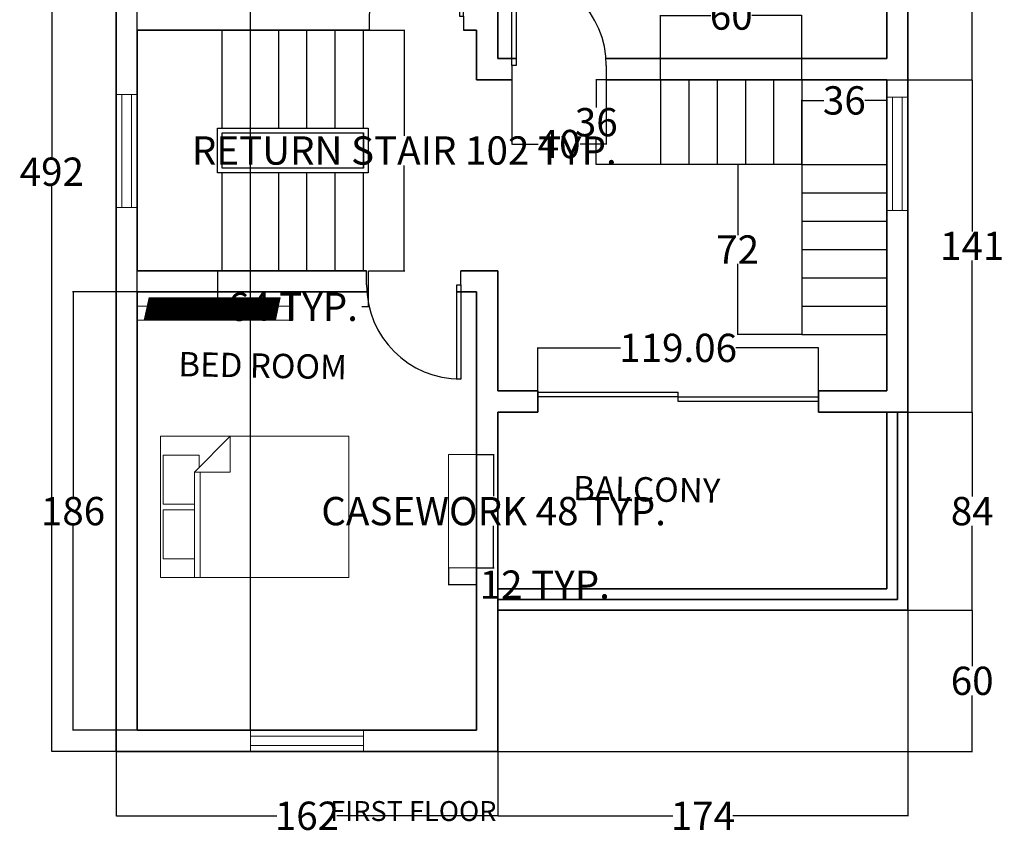
# Model space of a CAD drawing. Units: inches. Extents: x 424 to 1593, y 6 to 578.
# Tile 3 of 4: x 1175 to 1593, y 15 to 361. Entities that reach past the tile are written whole.
import ezdxf

# ---------------------------------------------------------------- set-up
doc = ezdxf.new("R2010")
doc.units = ezdxf.units.IN
doc.header["$MEASUREMENT"] = 0
for name, color, linetype, lineweight in [('A-ANNO-DIMS', 2, 'Continuous', 18), ('A-ANNO-TEXT', 7, 'Continuous', 25), ('A-AREA-IDEN', 7, 'Continuous', 18), ('A-DOOR', 3, 'Continuous', 25), ('A-FLOR-CASE', 9, 'Continuous', 18), ('A-FLOR-CASE-PATT', 252, 'Continuous', 13), ('A-FLOR-STRS', 7, 'Continuous', 25), ('A-FURN', 8, 'Continuous', 18), ('A-GLAZ', 4, 'Continuous', 18), ('A-WALL', 7, 'Continuous', 35)]:
    doc.layers.add(name, color=color, linetype=linetype, lineweight=lineweight)
doc.styles.get("Standard").update_dxf_attribs({"font": 'arial.ttf'})
doc.dimstyles.get("Standard").update_dxf_attribs({"dimtxt": 12, "dimasz": 0.18, "dimexe": 0.18, "dimexo": 0.0625, "dimgap": 0.09, "dimtad": 0, "dimtih": 1, "dimtoh": 1, "dimdec": 0, "dimzin": 0, "dimdsep": 46, "dimlunit": 3, "dimtxsty": 'Standard', "dimcen": 0.09, "dimadec": 0, "dimazin": 0, "dimtfac": 1, "dimtdec": 0, "dimtofl": 0, "dimtmove": 0, "dimatfit": 3, "dimfxl": 1, "dimtolj": 1, "dimtzin": 0, "dimarcsym": 0})

# ---------------------------------------------------------------- blocks, each defined once
blk = doc.blocks.new('*U3')
for p, q in [((0, 0), (0, -6)), ((-40, 0), (-40, -6))]:
    blk.add_line(p, q)
blk.add_lwpolyline([(0, 0), (0, 40), (-1.75, 40), (-1.75, 0)], close=True)
blk.add_arc((0, 0), 40, 90, 180)
blk = doc.blocks.new('*U4')
for p, q in [((-40, 0), (-40, 6)), ((0, 0), (0, 6))]:
    blk.add_line(p, q)
blk.add_lwpolyline([(0, 0), (0, -40), (-1.75, -40), (-1.75, 0)], close=True)
blk.add_arc((0, 0), 40, 180, 270)
blk = doc.blocks.new('*U6')
for p, q in [((0, 0), (0, -6)), ((40, 0), (40, -6))]:
    blk.add_line(p, q)
blk.add_lwpolyline([(0, 0), (0, 40), (1.75, 40), (1.75, 0)], close=True)
blk.add_arc((0, 0), 40, 0, 90)
blk = doc.blocks.new('Bed - Queen')
for p, q in [((0, -80.00003), (0, 0)), ((0, 0), (59.99999, 0)), ((59.99999, 0), (59.99999, -80.00003)), ((7.99999, -1.2), (28.79998, -1.2)), ((7.99999, -14.4), (7.99999, -1.2)), ((28.79998, -1.2), (28.79998, -14.4)), ((31.19999, -1.2), (51.99999, -1.2)), ((31.19999, -14.4), (31.19999, -1.2)), ((51.99999, -1.2), (51.99999, -16.4)), ((0, -14.4), (44.8, -14.4)), ((59.99999, -29.6), (44.8, -14.4)), ((44.8, -14.4), (44.8, -29.6)), ((51.99999, -16.4), (46.79936, -16.4)), ((44.8, -16.8), (0, -16.8)), ((44.8, -29.6), (59.99999, -29.6)), ((59.99999, -80.00003), (0, -80.00003))]:
    blk.add_line(p, q)
blk = doc.blocks.new('WIN-48IN')
for p, q in [((2.5, 48), (2.5, 0)), ((6.5, 48), (6.5, 0))]:
    blk.add_line(p, q)
blk.add_lwpolyline([(0, 48), (9, 48), (9, 0), (0, 0)], close=True)
blk = doc.blocks.new('STAIR-RETURN-102IN')
for p, q in [((2, 60.44), (2, 102)), ((14, 60.44), (14, 102)), ((26, 60.44), (26, 102)), ((38, 60.44), (38, 102)), ((50, 60.44), (50, 102)), ((62, 60.44), (62, 102)), ((2, 43.56), (2, 58.44)), ((62, 43.56), (62, 58.44)), ((2, 0), (2, 41.56)), ((14, 0), (14, 41.56)), ((26, 0), (26, 41.56)), ((38, 0), (38, 41.56)), ((50, 0), (50, 41.56)), ((62, 0), (62, 41.56))]:
    blk.add_line(p, q)
for points in [[(0, 60.44), (64, 60.44), (64, 41.56), (0, 41.56)], [(2, 58.44), (62, 58.44), (62, 43.56), (2, 43.56)]]:
    blk.add_lwpolyline(points, close=True)
blk = doc.blocks.new('CASEWORK-48X12')
blk.add_lwpolyline([(12, 48), (0, 48), (0, 0), (12, 0)], close=True)
blk = doc.blocks.new('*D18')
at = {"layer": 'A-ANNO-DIMS', "color": 0, "lineweight": -2, "transparency": 16777216}
for p, q in [((1368.79, 176.53), (1376.11, 176.53)), ((1375.93, 176.35), (1375.93, 158.83)), ((1375.93, 128.71), (1375.93, 146.23)), ((1368.79, 128.53), (1376.11, 128.53))]:
    blk.add_line(p, q, dxfattribs=at)
at = {"layer": 'A-ANNO-DIMS', "color": 0, "transparency": 16777216}
for points in [[(1375.9, 176.35), (1375.96, 176.35), (1375.93, 176.53)], [(1375.9, 128.71), (1375.96, 128.71), (1375.93, 128.53)]]:
    blk.add_solid(points, dxfattribs=at)
at = {"layer": 'Defpoints', "color": 0, "transparency": 16777216}
for p in [(1368.73, 176.53), (1375.93, 176.53), (1368.73, 128.53)]:
    blk.add_point(p, dxfattribs=at)
at = {"layer": 'A-ANNO-DIMS', "color": 0, "transparency": 16777216, "insert": (1375.93, 152.53), "char_height": 12, "attachment_point": 5}
blk.add_mtext('\\A1;CASEWORK 48 TYP.', dxfattribs=at)
blk = doc.blocks.new('*D19')
at = {"layer": 'A-ANNO-DIMS', "color": 0, "lineweight": -2, "transparency": 16777216}
for p, q in [((1356.73, 128.47), (1356.73, 121.15)), ((1368.73, 128.47), (1368.73, 121.15)), ((1356.91, 121.33), (1368.55, 121.33)), ((1368.73, 121.33), (1368.91, 121.33))]:
    blk.add_line(p, q, dxfattribs=at)
at = {"layer": 'A-ANNO-DIMS', "color": 0, "transparency": 16777216}
for points in [[(1356.91, 121.36), (1356.91, 121.3), (1356.73, 121.33)], [(1368.55, 121.36), (1368.55, 121.3), (1368.73, 121.33)]]:
    blk.add_solid(points, dxfattribs=at)
at = {"layer": 'Defpoints', "color": 0, "transparency": 16777216}
for p in [(1356.73, 128.53), (1368.73, 128.53), (1368.73, 121.33)]:
    blk.add_point(p, dxfattribs=at)
at = {"layer": 'A-ANNO-DIMS', "color": 0, "transparency": 16777216, "insert": (1397.64, 121.33), "char_height": 12, "attachment_point": 5}
blk.add_mtext('\\A1;12 TYP.', dxfattribs=at)
blk = doc.blocks.new('*D20')
at = {"layer": 'A-ANNO-DIMS', "color": 0, "lineweight": -2, "transparency": 16777216}
for p, q in [((1322.79, 356.53), (1338.21, 356.53)), ((1338.03, 356.35), (1338.03, 311.82)), ((1338.03, 254.71), (1338.03, 299.23)), ((1322.79, 254.53), (1338.21, 254.53))]:
    blk.add_line(p, q, dxfattribs=at)
at = {"layer": 'A-ANNO-DIMS', "color": 0, "transparency": 16777216}
for points in [[(1338, 356.35), (1338.06, 356.35), (1338.03, 356.53)], [(1338, 254.71), (1338.06, 254.71), (1338.03, 254.53)]]:
    blk.add_solid(points, dxfattribs=at)
at = {"layer": 'Defpoints', "color": 0, "transparency": 16777216}
for p in [(1322.73, 356.53), (1338.03, 356.53), (1322.73, 254.53)]:
    blk.add_point(p, dxfattribs=at)
at = {"layer": 'A-ANNO-DIMS', "color": 0, "transparency": 16777216, "insert": (1338.03, 305.53), "char_height": 12, "attachment_point": 5}
blk.add_mtext('\\A1;RETURN STAIR 102 TYP.', dxfattribs=at)
blk = doc.blocks.new('*D21')
at = {"layer": 'A-ANNO-DIMS', "color": 0, "lineweight": -2, "transparency": 16777216}
for p, q in [((1258.73, 254.47), (1258.73, 239.05)), ((1322.73, 254.47), (1322.73, 239.05)), ((1258.91, 239.23), (1261.4, 239.23)), ((1322.55, 239.23), (1320.06, 239.23))]:
    blk.add_line(p, q, dxfattribs=at)
at = {"layer": 'A-ANNO-DIMS', "color": 0, "transparency": 16777216}
for points in [[(1258.91, 239.26), (1258.91, 239.2), (1258.73, 239.23)], [(1322.55, 239.26), (1322.55, 239.2), (1322.73, 239.23)]]:
    blk.add_solid(points, dxfattribs=at)
at = {"layer": 'Defpoints', "color": 0, "transparency": 16777216}
for p in [(1258.73, 254.53), (1322.73, 254.53), (1322.73, 239.23)]:
    blk.add_point(p, dxfattribs=at)
at = {"layer": 'A-ANNO-DIMS', "color": 0, "transparency": 16777216, "insert": (1290.73, 239.23), "char_height": 12, "attachment_point": 5}
blk.add_mtext('\\A1;64 TYP.', dxfattribs=at)
blk = doc.blocks.new('*D49')
at = {"layer": 'A-ANNO-DIMS', "color": 0, "lineweight": -2, "transparency": 16777216}
for p, q in [((1215.66, 542.53), (1188.3, 542.53)), ((1188.48, 542.35), (1188.48, 302.75)), ((1188.48, 50.71), (1188.48, 290.31)), ((1215.66, 50.53), (1188.3, 50.53))]:
    blk.add_line(p, q, dxfattribs=at)
at = {"layer": 'A-ANNO-DIMS', "color": 0, "transparency": 16777216}
for points in [[(1188.45, 542.35), (1188.51, 542.35), (1188.48, 542.53)], [(1188.45, 50.71), (1188.51, 50.71), (1188.48, 50.53)]]:
    blk.add_solid(points, dxfattribs=at)
at = {"layer": 'Defpoints', "color": 0, "transparency": 16777216}
for p in [(1188.48, 542.53), (1215.73, 542.53), (1215.73, 50.53)]:
    blk.add_point(p, dxfattribs=at)
at = {"layer": 'A-ANNO-DIMS', "color": 0, "transparency": 16777216, "insert": (1188.48, 296.53), "char_height": 12, "attachment_point": 5}
blk.add_mtext('\\A1;492', dxfattribs=at)
blk = doc.blocks.new('*D50')
at = {"layer": 'A-ANNO-DIMS', "color": 0, "lineweight": -2, "transparency": 16777216}
for p, q in [((1215.73, 50.47), (1215.73, 23.1)), ((1377.73, 50.47), (1377.73, 23.1)), ((1215.91, 23.28), (1284.01, 23.28)), ((1377.55, 23.28), (1309.45, 23.28))]:
    blk.add_line(p, q, dxfattribs=at)
at = {"layer": 'A-ANNO-DIMS', "color": 0, "transparency": 16777216}
for points in [[(1215.91, 23.31), (1215.91, 23.25), (1215.73, 23.28)], [(1377.55, 23.31), (1377.55, 23.25), (1377.73, 23.28)]]:
    blk.add_solid(points, dxfattribs=at)
at = {"layer": 'Defpoints', "color": 0, "transparency": 16777216}
for p in [(1215.73, 50.53), (1377.73, 50.53), (1377.73, 23.28)]:
    blk.add_point(p, dxfattribs=at)
at = {"layer": 'A-ANNO-DIMS', "color": 0, "transparency": 16777216, "insert": (1296.73, 23.28), "char_height": 12, "attachment_point": 5}
blk.add_mtext('\\A1;162', dxfattribs=at)
blk = doc.blocks.new('*D51')
at = {"layer": 'A-ANNO-DIMS', "color": 0, "lineweight": -2, "transparency": 16777216}
for p, q in [((1377.73, 110.47), (1377.73, 23.1)), ((1551.73, 110.47), (1551.73, 23.1)), ((1377.91, 23.28), (1451.97, 23.28)), ((1551.55, 23.28), (1477.48, 23.28))]:
    blk.add_line(p, q, dxfattribs=at)
at = {"layer": 'A-ANNO-DIMS', "color": 0, "transparency": 16777216}
for points in [[(1377.91, 23.31), (1377.91, 23.25), (1377.73, 23.28)], [(1551.55, 23.31), (1551.55, 23.25), (1551.73, 23.28)]]:
    blk.add_solid(points, dxfattribs=at)
at = {"layer": 'Defpoints', "color": 0, "transparency": 16777216}
for p in [(1377.73, 110.53), (1551.73, 110.53), (1551.73, 23.28)]:
    blk.add_point(p, dxfattribs=at)
at = {"layer": 'A-ANNO-DIMS', "color": 0, "transparency": 16777216, "insert": (1464.73, 23.28), "char_height": 12, "attachment_point": 5}
blk.add_mtext('\\A1;174', dxfattribs=at)
blk = doc.blocks.new('*D52')
at = {"layer": 'A-ANNO-DIMS', "color": 0, "lineweight": -2, "transparency": 16777216}
for p, q in [((1224.66, 245.53), (1197.3, 245.53)), ((1197.48, 245.35), (1197.48, 158.75)), ((1197.48, 59.71), (1197.48, 146.31)), ((1224.66, 59.53), (1197.3, 59.53))]:
    blk.add_line(p, q, dxfattribs=at)
at = {"layer": 'A-ANNO-DIMS', "color": 0, "transparency": 16777216}
for points in [[(1197.45, 245.35), (1197.51, 245.35), (1197.48, 245.53)], [(1197.45, 59.71), (1197.51, 59.71), (1197.48, 59.53)]]:
    blk.add_solid(points, dxfattribs=at)
at = {"layer": 'Defpoints', "color": 0, "transparency": 16777216}
for p in [(1197.48, 245.53), (1224.73, 245.53), (1224.73, 59.53)]:
    blk.add_point(p, dxfattribs=at)
at = {"layer": 'A-ANNO-DIMS', "color": 0, "transparency": 16777216, "insert": (1197.48, 152.53), "char_height": 12, "attachment_point": 5}
blk.add_mtext('\\A1;186', dxfattribs=at)
blk = doc.blocks.new('*D55')
at = {"layer": 'A-ANNO-DIMS', "color": 0, "lineweight": -2, "transparency": 16777216}
for p, q in [((1551.79, 110.53), (1579.16, 110.53)), ((1578.98, 110.35), (1578.98, 86.75)), ((1578.98, 50.71), (1578.98, 74.31)), ((1377.79, 50.53), (1579.16, 50.53))]:
    blk.add_line(p, q, dxfattribs=at)
at = {"layer": 'A-ANNO-DIMS', "color": 0, "transparency": 16777216}
for points in [[(1578.95, 110.35), (1579.01, 110.35), (1578.98, 110.53)], [(1578.95, 50.71), (1579.01, 50.71), (1578.98, 50.53)]]:
    blk.add_solid(points, dxfattribs=at)
at = {"layer": 'Defpoints', "color": 0, "transparency": 16777216}
for p in [(1551.73, 110.53), (1578.98, 110.53), (1377.73, 50.53)]:
    blk.add_point(p, dxfattribs=at)
at = {"layer": 'A-ANNO-DIMS', "color": 0, "transparency": 16777216, "insert": (1578.98, 80.53), "char_height": 12, "attachment_point": 5}
blk.add_mtext('\\A1;60', dxfattribs=at)
blk = doc.blocks.new('*D56')
at = {"layer": 'A-ANNO-DIMS', "color": 0, "lineweight": -2, "transparency": 16777216}
for p, q in [((1551.79, 194.53), (1579.16, 194.53)), ((1578.98, 194.35), (1578.98, 158.75)), ((1578.98, 110.71), (1578.98, 146.31)), ((1551.79, 110.53), (1579.16, 110.53))]:
    blk.add_line(p, q, dxfattribs=at)
at = {"layer": 'A-ANNO-DIMS', "color": 0, "transparency": 16777216}
for points in [[(1578.95, 194.35), (1579.01, 194.35), (1578.98, 194.53)], [(1578.95, 110.71), (1579.01, 110.71), (1578.98, 110.53)]]:
    blk.add_solid(points, dxfattribs=at)
at = {"layer": 'Defpoints', "color": 0, "transparency": 16777216}
for p in [(1551.73, 194.53), (1578.98, 194.53), (1551.73, 110.53)]:
    blk.add_point(p, dxfattribs=at)
at = {"layer": 'A-ANNO-DIMS', "color": 0, "transparency": 16777216, "insert": (1578.98, 152.53), "char_height": 12, "attachment_point": 5}
blk.add_mtext('\\A1;84', dxfattribs=at)
blk = doc.blocks.new('*D57')
at = {"layer": 'A-ANNO-DIMS', "color": 0, "lineweight": -2, "transparency": 16777216}
for p, q in [((1542.79, 335.53), (1579.16, 335.53)), ((1578.98, 335.35), (1578.98, 271.14)), ((1578.98, 194.71), (1578.98, 258.92)), ((1551.79, 194.53), (1579.16, 194.53))]:
    blk.add_line(p, q, dxfattribs=at)
at = {"layer": 'A-ANNO-DIMS', "color": 0, "transparency": 16777216}
for points in [[(1578.95, 335.35), (1579.01, 335.35), (1578.98, 335.53)], [(1578.95, 194.71), (1579.01, 194.71), (1578.98, 194.53)]]:
    blk.add_solid(points, dxfattribs=at)
at = {"layer": 'Defpoints', "color": 0, "transparency": 16777216}
for p in [(1542.73, 335.53), (1578.98, 335.53), (1551.73, 194.53)]:
    blk.add_point(p, dxfattribs=at)
at = {"layer": 'A-ANNO-DIMS', "color": 0, "transparency": 16777216, "insert": (1578.98, 265.03), "char_height": 12, "attachment_point": 5}
blk.add_mtext('\\A1;141', dxfattribs=at)
blk = doc.blocks.new('*D58')
at = {"layer": 'A-ANNO-DIMS', "color": 0, "lineweight": -2, "transparency": 16777216}
for p, q in [((1551.79, 473.53), (1579.16, 473.53)), ((1578.98, 473.35), (1578.98, 410.75)), ((1578.98, 335.71), (1578.98, 398.31)), ((1542.79, 335.53), (1579.16, 335.53))]:
    blk.add_line(p, q, dxfattribs=at)
at = {"layer": 'A-ANNO-DIMS', "color": 0, "transparency": 16777216}
for points in [[(1578.95, 473.35), (1579.01, 473.35), (1578.98, 473.53)], [(1578.95, 335.71), (1579.01, 335.71), (1578.98, 335.53)]]:
    blk.add_solid(points, dxfattribs=at)
at = {"layer": 'Defpoints', "color": 0, "transparency": 16777216}
for p in [(1551.73, 473.53), (1578.98, 473.53), (1542.73, 335.53)]:
    blk.add_point(p, dxfattribs=at)
at = {"layer": 'A-ANNO-DIMS', "color": 0, "transparency": 16777216, "insert": (1578.98, 404.53), "char_height": 12, "attachment_point": 5}
blk.add_mtext('\\A1;138', dxfattribs=at)
blk = doc.blocks.new('*D62')
at = {"layer": 'A-ANNO-DIMS', "color": 0, "lineweight": -2, "transparency": 16777216}
for p, q in [((1394.67, 194.59), (1394.67, 221.96)), ((1394.85, 221.78), (1429.78, 221.78)), ((1513.56, 221.78), (1478.64, 221.78)), ((1513.74, 194.59), (1513.74, 221.96))]:
    blk.add_line(p, q, dxfattribs=at)
at = {"layer": 'A-ANNO-DIMS', "color": 0, "transparency": 16777216}
for points in [[(1394.85, 221.81), (1394.85, 221.75), (1394.67, 221.78)], [(1513.56, 221.81), (1513.56, 221.75), (1513.74, 221.78)]]:
    blk.add_solid(points, dxfattribs=at)
at = {"layer": 'Defpoints', "color": 0, "transparency": 16777216}
for p in [(1513.74, 221.78), (1394.67, 194.53), (1513.74, 194.53)]:
    blk.add_point(p, dxfattribs=at)
at = {"layer": 'A-ANNO-DIMS', "color": 0, "transparency": 16777216, "insert": (1454.21, 221.78), "char_height": 12, "attachment_point": 5}
blk.add_mtext('\\A1;119.06', dxfattribs=at)
blk = doc.blocks.new('*D63')
at = {"layer": 'A-ANNO-DIMS', "color": 0, "lineweight": -2, "transparency": 16777216}
for p, q in [((1224.73, 59.59), (1224.73, 569.96)), ((1224.91, 569.78), (1239.79, 569.78)), ((1272.55, 569.78), (1257.67, 569.78)), ((1272.73, 59.59), (1272.73, 569.96))]:
    blk.add_line(p, q, dxfattribs=at)
at = {"layer": 'A-ANNO-DIMS', "color": 0, "transparency": 16777216}
for points in [[(1224.91, 569.81), (1224.91, 569.75), (1224.73, 569.78)], [(1272.55, 569.81), (1272.55, 569.75), (1272.73, 569.78)]]:
    blk.add_solid(points, dxfattribs=at)
at = {"layer": 'Defpoints', "color": 0, "transparency": 16777216}
for p in [(1272.73, 569.78), (1224.73, 59.53), (1272.73, 59.53)]:
    blk.add_point(p, dxfattribs=at)
at = {"layer": 'A-ANNO-DIMS', "color": 0, "transparency": 16777216, "insert": (1248.73, 569.78), "char_height": 12, "attachment_point": 5}
blk.add_mtext('\\A1;48', dxfattribs=at)
blk = doc.blocks.new('*D65')
at = {"layer": 'A-ANNO-DIMS', "color": 0, "lineweight": -2, "transparency": 16777216}
for p, q in [((1506.73, 299.59), (1506.73, 326.96)), ((1506.91, 326.78), (1516.05, 326.78)), ((1542.55, 326.78), (1533.4, 326.78)), ((1542.73, 299.59), (1542.73, 326.96))]:
    blk.add_line(p, q, dxfattribs=at)
at = {"layer": 'A-ANNO-DIMS', "color": 0, "transparency": 16777216}
for points in [[(1506.91, 326.81), (1506.91, 326.75), (1506.73, 326.78)], [(1542.55, 326.81), (1542.55, 326.75), (1542.73, 326.78)]]:
    blk.add_solid(points, dxfattribs=at)
at = {"layer": 'Defpoints', "color": 0, "transparency": 16777216}
for p in [(1542.73, 326.78), (1506.73, 299.53), (1542.73, 299.53)]:
    blk.add_point(p, dxfattribs=at)
at = {"layer": 'A-ANNO-DIMS', "color": 0, "transparency": 16777216, "insert": (1524.73, 326.78), "char_height": 12, "attachment_point": 5}
blk.add_mtext('\\A1;36', dxfattribs=at)
blk = doc.blocks.new('*D66')
at = {"layer": 'A-ANNO-DIMS', "color": 0, "lineweight": -2, "transparency": 16777216}
for p, q in [((1506.66, 299.53), (1479.3, 299.53)), ((1479.48, 299.35), (1479.48, 269.64)), ((1479.48, 227.71), (1479.48, 257.42)), ((1506.66, 227.53), (1479.3, 227.53))]:
    blk.add_line(p, q, dxfattribs=at)
at = {"layer": 'A-ANNO-DIMS', "color": 0, "transparency": 16777216}
for points in [[(1479.45, 299.35), (1479.51, 299.35), (1479.48, 299.53)], [(1479.45, 227.71), (1479.51, 227.71), (1479.48, 227.53)]]:
    blk.add_solid(points, dxfattribs=at)
at = {"layer": 'Defpoints', "color": 0, "transparency": 16777216}
for p in [(1479.48, 299.53), (1506.73, 299.53), (1506.73, 227.53)]:
    blk.add_point(p, dxfattribs=at)
at = {"layer": 'A-ANNO-DIMS', "color": 0, "transparency": 16777216, "insert": (1479.48, 263.53), "char_height": 12, "attachment_point": 5}
blk.add_mtext('\\A1;72', dxfattribs=at)
blk = doc.blocks.new('*D67')
at = {"layer": 'A-ANNO-DIMS', "color": 0, "lineweight": -2, "transparency": 16777216}
for p, q in [((1446.73, 335.59), (1446.73, 362.96)), ((1446.91, 362.78), (1468.03, 362.78)), ((1506.55, 362.78), (1485.42, 362.78)), ((1506.73, 335.59), (1506.73, 362.96))]:
    blk.add_line(p, q, dxfattribs=at)
at = {"layer": 'A-ANNO-DIMS', "color": 0, "transparency": 16777216}
for points in [[(1446.91, 362.81), (1446.91, 362.75), (1446.73, 362.78)], [(1506.55, 362.81), (1506.55, 362.75), (1506.73, 362.78)]]:
    blk.add_solid(points, dxfattribs=at)
at = {"layer": 'Defpoints', "color": 0, "transparency": 16777216}
for p in [(1506.73, 362.78), (1446.73, 335.53), (1506.73, 335.53)]:
    blk.add_point(p, dxfattribs=at)
at = {"layer": 'A-ANNO-DIMS', "color": 0, "transparency": 16777216, "insert": (1476.73, 362.78), "char_height": 12, "attachment_point": 5}
blk.add_mtext('\\A1;60', dxfattribs=at)
blk = doc.blocks.new('*D68')
at = {"layer": 'A-ANNO-DIMS', "color": 0, "lineweight": -2, "transparency": 16777216}
for p, q in [((1446.66, 335.53), (1419.3, 335.53)), ((1419.48, 335.35), (1419.48, 323.75)), ((1419.48, 299.71), (1419.48, 311.31)), ((1446.66, 299.53), (1419.3, 299.53))]:
    blk.add_line(p, q, dxfattribs=at)
at = {"layer": 'A-ANNO-DIMS', "color": 0, "transparency": 16777216}
for points in [[(1419.45, 335.35), (1419.51, 335.35), (1419.48, 335.53)], [(1419.45, 299.71), (1419.51, 299.71), (1419.48, 299.53)]]:
    blk.add_solid(points, dxfattribs=at)
at = {"layer": 'Defpoints', "color": 0, "transparency": 16777216}
for p in [(1419.48, 335.53), (1446.73, 335.53), (1446.73, 299.53)]:
    blk.add_point(p, dxfattribs=at)
at = {"layer": 'A-ANNO-DIMS', "color": 0, "transparency": 16777216, "insert": (1419.48, 317.53), "char_height": 12, "attachment_point": 5}
blk.add_mtext('\\A1;36', dxfattribs=at)
blk = doc.blocks.new('*D71')
at = {"layer": 'A-ANNO-DIMS', "color": 0, "lineweight": -2, "transparency": 16777216}
for p, q in [((1383.72, 335.47), (1383.72, 308.1)), ((1423.72, 335.47), (1423.72, 308.1)), ((1383.9, 308.28), (1394.81, 308.28)), ((1423.54, 308.28), (1412.62, 308.28))]:
    blk.add_line(p, q, dxfattribs=at)
at = {"layer": 'A-ANNO-DIMS', "color": 0, "transparency": 16777216}
for points in [[(1383.9, 308.31), (1383.9, 308.25), (1383.72, 308.28)], [(1423.54, 308.31), (1423.54, 308.25), (1423.72, 308.28)]]:
    blk.add_solid(points, dxfattribs=at)
at = {"layer": 'Defpoints', "color": 0, "transparency": 16777216}
for p in [(1383.72, 335.53), (1423.72, 335.53), (1383.72, 308.28)]:
    blk.add_point(p, dxfattribs=at)
at = {"layer": 'A-ANNO-DIMS', "color": 0, "transparency": 16777216, "insert": (1403.72, 308.28), "char_height": 12, "attachment_point": 5}
blk.add_mtext('\\A1;40', dxfattribs=at)

msp = doc.modelspace()

# ---------------------------------------------------------------- hatches: boundary and pattern name
at = {"layer": 'A-FLOR-CASE-PATT'}
h = msp.add_hatch(dxfattribs=at)
h.set_pattern_fill('ANSI31', color=256, scale=1.232385, angle=33.269, style=0)
h.paths.add_polyline_path([(1227.5677, 233.5296), (1283.5157, 233.5296), (1285.5139, 243.1524), (1229.5659, 243.1524)])

# ---------------------------------------------------------------- linework, layer by layer
at = {"layer": 'A-DOOR'}
for p, q in [((1394.6736, 203.0296), (1454.206, 203.0296)), ((1454.206, 201.0296), (1394.6736, 201.0296)), ((1454.206, 199.0296), (1454.206, 203.0296)), ((1454.206, 201.0296), (1513.7383, 201.0296)), ((1513.7383, 199.0296), (1454.206, 199.0296))]:
    msp.add_line(p, q, dxfattribs=at)
at = {"layer": 'A-FLOR-CASE'}
msp.add_line((1290.7275, 239.5296), (1224.7275, 239.5296), dxfattribs=at)
msp.add_lwpolyline([(1224.7275, 245.5296), (1290.7275, 245.5296), (1290.7275, 233.5296), (1224.7275, 233.5296)], close=True, dxfattribs=at)
at = {"layer": 'A-FLOR-STRS'}
for p, q in [((1446.7275, 335.5296), (1446.7275, 299.5296)), ((1458.7275, 335.5296), (1458.7275, 299.5296)), ((1470.7275, 335.5296), (1470.7275, 299.5296)), ((1482.7275, 335.5296), (1482.7275, 299.5296)), ((1494.7275, 335.5296), (1494.7275, 299.5296)), ((1542.7275, 335.5296), (1506.7275, 335.5296)), ((1506.7275, 335.5296), (1506.7275, 299.5296)), ((1542.7275, 299.5296), (1542.7275, 335.5296)), ((1506.7275, 299.5296), (1446.7275, 299.5296)), ((1506.7275, 299.5296), (1506.7275, 227.5296)), ((1506.7275, 299.5296), (1542.7275, 299.5296)), ((1506.7275, 287.5296), (1542.7275, 287.5296)), ((1506.7275, 275.5296), (1542.7275, 275.5296)), ((1506.7275, 263.5296), (1542.7275, 263.5296)), ((1506.7275, 251.5296), (1542.7275, 251.5296)), ((1506.7275, 239.5296), (1542.7275, 239.5296)), ((1506.7275, 227.5296), (1542.7275, 227.5296))]:
    msp.add_line(p, q, dxfattribs=at)
at = {"layer": 'A-WALL'}
for p, q in [((1377.7275, 464.5296), (1377.7275, 344.5296)), ((1542.7275, 464.5296), (1542.7275, 344.5296)), ((1224.7275, 356.5296), (1323.1588, 356.5296)), ((1224.7275, 254.5296), (1224.7275, 356.5296)), ((1363.1588, 356.5296), (1368.7275, 356.5296)), ((1368.7275, 356.5296), (1368.7275, 335.5296)), ((1377.7275, 344.5296), (1385.4659, 344.5296)), ((1423.6032, 344.5296), (1542.7275, 344.5296)), ((1368.7275, 335.5296), (1383.7159, 335.5296)), ((1383.7159, 335.5296), (1377.7159, 335.5296)), ((1423.7159, 335.5296), (1542.7275, 335.5296)), ((1542.7275, 335.5296), (1542.7275, 203.5296)), ((1224.7275, 254.5296), (1322.0093, 254.5296)), ((1362.0093, 254.5296), (1377.7275, 254.5296)), ((1377.7275, 254.5296), (1377.7275, 203.5296)), ((1224.7275, 59.5296), (1224.7275, 245.5296)), ((1224.7275, 245.5296), (1322.1219, 245.5296)), ((1360.2593, 245.5296), (1368.7275, 245.5296)), ((1368.7275, 245.5296), (1368.7275, 59.5296)), ((1377.7275, 203.5296), (1394.6736, 203.5296)), ((1394.6736, 203.5296), (1394.6736, 194.5296)), ((1513.7383, 203.5296), (1513.7383, 194.5296)), ((1513.7383, 203.5296), (1542.7275, 203.5296)), ((1377.7275, 194.5296), (1394.6736, 194.5296)), ((1377.7275, 194.5296), (1377.7275, 110.5296)), ((1513.7383, 194.5296), (1551.7275, 194.5296)), ((1542.7275, 194.5296), (1542.7275, 119.5296)), ((1547.2275, 115.0296), (1547.2275, 194.5296)), ((1377.7275, 119.5296), (1542.7275, 119.5296)), ((1547.2275, 115.0296), (1377.7275, 115.0296)), ((1377.7275, 110.5296), (1551.7275, 110.5296)), ((1377.7275, 110.5296), (1377.7275, 50.5296)), ((1368.7275, 59.5296), (1224.7275, 59.5296))]:
    msp.add_line(p, q, dxfattribs=at)
for points in [[(1377.7275, 50.5296), (1215.7275, 50.5296), (1215.7275, 542.5296), (1377.7275, 542.5296)], [(1377.7275, 50.5296), (1215.7275, 50.5296), (1215.7275, 542.5296), (1377.7275, 542.5296)], [(1551.7275, 473.5296), (1551.7275, 110.5296)], [(1542.7275, 464.5296), (1542.7275, 344.5296)], [(1224.7275, 254.5296), (1224.7275, 356.5296)], [(1542.7275, 335.5296), (1542.7275, 203.5296)], [(1368.7275, 59.5296), (1224.7275, 59.5296), (1224.7275, 245.5296)], [(1542.7275, 194.5296), (1542.7275, 119.5296)], [(1551.7275, 194.5296), (1551.7275, 110.5296)]]:
    msp.add_lwpolyline(points, dxfattribs=at)

# ---------------------------------------------------------------- block references
at = {"layer": 'A-DOOR'}
for name, p in [('*U3', (1363.1588, 362.5296)), ('*U6', (1383.7159, 341.5296)), ('*U4', (1362.0093, 248.5296))]:
    msp.add_blockref(name, p, dxfattribs=at)
at = {"layer": 'A-FLOR-CASE'}
msp.add_blockref('CASEWORK-48X12', (1356.7276, 128.5295), dxfattribs=at)
at = {"layer": 'A-FLOR-STRS'}
msp.add_blockref('STAIR-RETURN-102IN', (1258.7276, 254.53), dxfattribs=at)
at = {"layer": 'A-FURN', "rotation": 90}
msp.add_blockref('Bed - Queen', (1234.5518, 124.3181), dxfattribs=at)
at = {"layer": 'A-GLAZ'}
for p in [(1215.7276, 281.28), (1542.7276, 280.1297)]:
    msp.add_blockref('WIN-48IN', p, dxfattribs=at)
at = {"layer": 'A-GLAZ', "rotation": 89.99999999999996}
msp.add_blockref('WIN-48IN', (1320.7276, 50.5297), dxfattribs=at)

# ---------------------------------------------------------------- texts
at = {"layer": 'A-ANNO-TEXT'}
msp.add_text('FIRST FLOOR', height=8.45662, dxfattribs=at).set_placement((1306.6053, 21.0429))
at = {"layer": 'A-AREA-IDEN'}
for s, p in [('BED ROOM', (1242.0717, 209.7911)), ('BALCONY  ', (1409.5761, 157.2153))]:
    msp.add_text(s, height=10.30671, rotation=358.915866, dxfattribs=at).set_placement(p)

# ---------------------------------------------------------------- dimensions: what is measured, and where the dimension line sits
at = {"layer": 'A-ANNO-DIMS'}
for base, p1, p2, override, picture, middle in [((1272.7275, 569.7796), (1224.7275, 59.5296), (1272.7275, 59.5296), {"dimdec": 0, "dimlfac": 1, "dimrnd": 0, "dimzin": 0, "dimdsep": 46, "dimlunit": 2}, '*D63', (1248.7275, 569.7796)), ((1506.7275, 362.7796), (1446.7275, 335.5296), (1506.7275, 335.5296), {"dimdec": 0, "dimlfac": 1, "dimrnd": 0, "dimzin": 0, "dimdsep": 46, "dimlunit": 2}, '*D67', (1476.7275, 362.7796)), ((1542.7275, 326.7796), (1506.7275, 299.5296), (1542.7275, 299.5296), {"dimdec": 0, "dimlfac": 1, "dimrnd": 0, "dimzin": 0, "dimdsep": 46, "dimlunit": 2}, '*D65', (1524.7275, 326.7796)), ((1513.7383, 221.7796), (1394.6736, 194.5296), (1513.7383, 194.5296), {"dimdec": 2, "dimlfac": 1, "dimrnd": 0, "dimzin": 0, "dimdsep": 46, "dimlunit": 2}, '*D62', (1454.206, 221.7796)), ((1551.7275, 23.2796), (1377.7275, 110.5296), (1551.7275, 110.5296), {"dimdec": 0, "dimlfac": 1, "dimrnd": 0, "dimzin": 0, "dimdsep": 46, "dimlunit": 2}, '*D51', (1464.7275, 23.2796)), ((1377.7275, 23.2796), (1215.7275, 50.5296), (1377.7275, 50.5296), {"dimdec": 0, "dimlfac": 1, "dimrnd": 0, "dimzin": 0, "dimdsep": 46, "dimlunit": 2}, '*D50', (1296.7275, 23.2796))]:
    dim = msp.add_linear_dim(base=base, p1=p1, p2=p2, dimstyle='Standard', override=override, dxfattribs=at)
    dim.commit()
    dim.dimension.update_dxf_attribs({"geometry": picture, "text_midpoint": middle})
for base, p1, p2, angle, picture, middle in [((1188.4775, 542.5296), (1215.7275, 50.5296), (1215.7275, 542.5296), 90, '*D49', (1188.4775, 296.5296)), ((1578.9775, 473.5296), (1542.7275, 335.5296), (1551.7275, 473.5296), 90, '*D58', (1578.9775, 404.5296)), ((1383.7159, 308.2796), (1423.7159, 335.5296), (1383.7159, 335.5296), 180, '*D71', (1403.7159, 308.2796)), ((1419.4775, 335.5296), (1446.7275, 299.5296), (1446.7275, 335.5296), 90, '*D68', (1419.4775, 317.5296)), ((1578.9775, 335.5296), (1551.7275, 194.5296), (1542.7275, 335.5296), 90, '*D57', (1578.9775, 265.0296)), ((1479.4775, 299.5296), (1506.7275, 227.5296), (1506.7275, 299.5296), 90, '*D66', (1479.4775, 263.5296)), ((1197.4775, 245.5296), (1224.7275, 59.5296), (1224.7275, 245.5296), 90, '*D52', (1197.4775, 152.5296)), ((1578.9775, 194.5296), (1551.7275, 110.5296), (1551.7275, 194.5296), 90, '*D56', (1578.9775, 152.5296)), ((1578.9775, 110.5296), (1377.7275, 50.5296), (1551.7275, 110.5296), 90, '*D55', (1578.9775, 80.5296))]:
    dim = msp.add_linear_dim(base=base, p1=p1, p2=p2, angle=angle, dimstyle='Standard', override={"dimdec": 0, "dimlfac": 1, "dimrnd": 0, "dimzin": 0, "dimdsep": 46, "dimlunit": 2}, dxfattribs=at)
    dim.commit()
    dim.dimension.update_dxf_attribs({"geometry": picture, "text_midpoint": middle})
for base, p1, p2, text, picture, middle in [((1338.0275, 356.5296), (1322.7275, 254.5296), (1322.7275, 356.5296), 'RETURN STAIR <> TYP.', '*D20', (1338.0275, 305.5296)), ((1375.9275, 176.5296), (1368.7275, 128.5296), (1368.7275, 176.5296), 'CASEWORK <> TYP.', '*D18', (1375.9275, 152.5296))]:
    dim = msp.add_linear_dim(base=base, p1=p1, p2=p2, angle=90, text=text, dimstyle='Standard', override={"dimdec": 0, "dimlfac": 1, "dimrnd": 0, "dimzin": 0, "dimdsep": 46, "dimlunit": 2}, dxfattribs=at)
    dim.commit()
    dim.dimension.update_dxf_attribs({"geometry": picture, "text_midpoint": middle})
for base, p1, p2, picture, middle in [((1322.7275, 239.2296), (1258.7275, 254.5296), (1322.7275, 254.5296), '*D21', (1290.7275, 239.2296)), ((1368.7275, 121.3296), (1356.7275, 128.5296), (1368.7275, 128.5296), '*D19', (1397.6387, 121.3296))]:
    dim = msp.add_linear_dim(base=base, p1=p1, p2=p2, text='<> TYP.', dimstyle='Standard', override={"dimdec": 0, "dimlfac": 1, "dimrnd": 0, "dimzin": 0, "dimdsep": 46, "dimlunit": 2}, dxfattribs=at)
    dim.commit()
    dim.dimension.update_dxf_attribs({"geometry": picture, "text_midpoint": middle})

doc.saveas('drawing.dxf')
